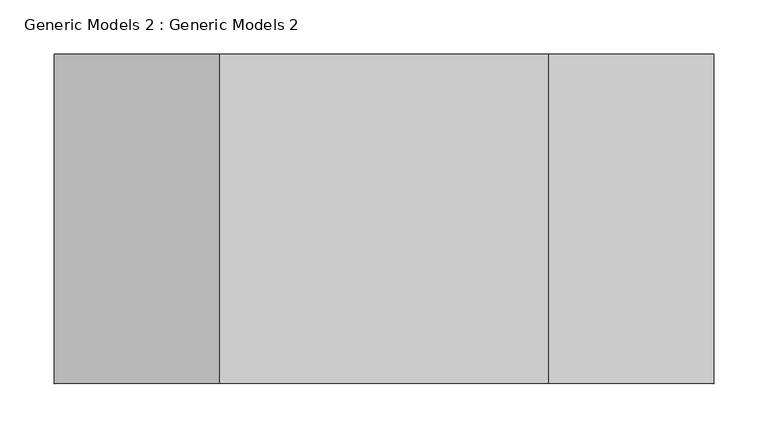
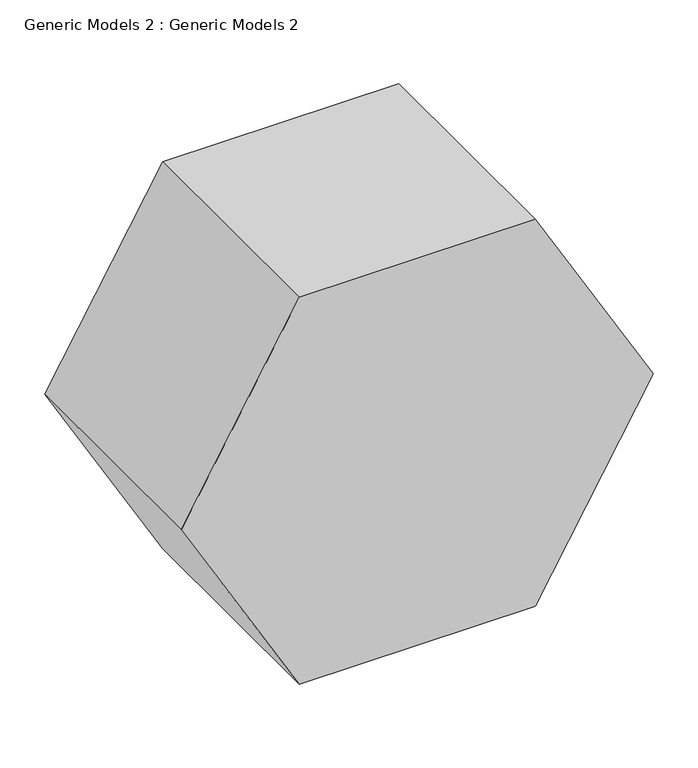
"""IFC4 building model written with IfcOpenShell, lengths in millimetres: proxy geometry, Generic Models 2 : Generic Models 2."""

from ifc_helpers import new_model, si_unit, frame, origin, place, context, project, spatial, polyline, outline, extrude, source, transform, mapped, element, save


def generic_models_2_generic_models_2_4eaefd90(model_context):
    return source(origin(), model_context, "Body", "SweptSolid", [
        extrude(outline(polyline([(850.692133, -5446.807544), (586.7275899, -5599.207544), (322.7630468, -5446.807544), (322.7630468, -5142.007544), (586.7275899, -4989.607544), (850.692133, -5142.007544), (850.692133, -5446.807544)])), frame((0.0, -8675.4830082, 0.0), z_axis=(0.0, 1.0, 0.0), x_axis=(0.0, 0.0, 1.0)), (0.0, 0.0, 1.0), 304.8),
    ])


if __name__ == "__main__":
    model = new_model("IFC4")
    model_context = context("Model", 3, world=origin())
    ifc_project = project(units=[si_unit("LENGTHUNIT", "METRE", prefix="MILLI")], contexts=[model_context])
    site = spatial("IfcSite", under=ifc_project)
    building = spatial("IfcBuilding", under=site)
    placement = place(None, origin())
    generic_models_2_generic_models_2_shape = generic_models_2_generic_models_2_4eaefd90(model_context)
    element("IfcBuildingElementProxy", 1, Name="Generic Models 2 : Generic Models 2", ObjectType="Generic Models 2 : Generic Models 2", at=placement, inside=building, context=model_context, shape_type="MappedRepresentation", body=[
        mapped(generic_models_2_generic_models_2_shape, transform((0.0, 0.0, 0.0), x_axis=(1.0, 0.0, 0.0), y_axis=(0.0, 1.0, 0.0), z_axis=(0.0, 0.0, 1.0))),
    ])
    save(model, "model.ifc")

# Revit data of these elements
# Element 1 (IfcBuildingElementProxy, "Generic Models 2 : Generic Models 2")
#   Materials on its faces: "Wood - Stained"
# Materials
#   "Wood - Stained": class "Wood", colour RGB 224 178 126, transparency 0, Cost = 0
